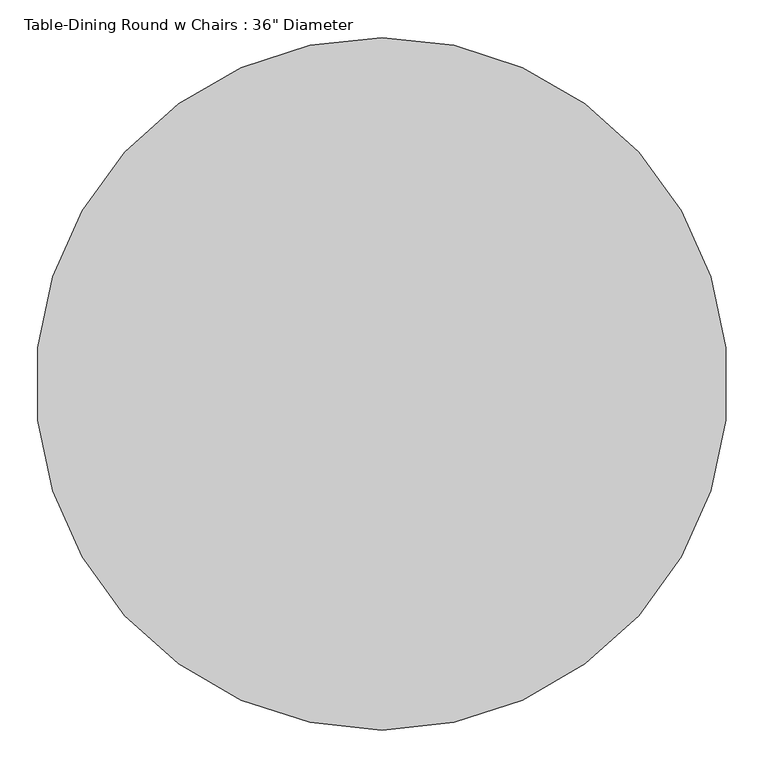
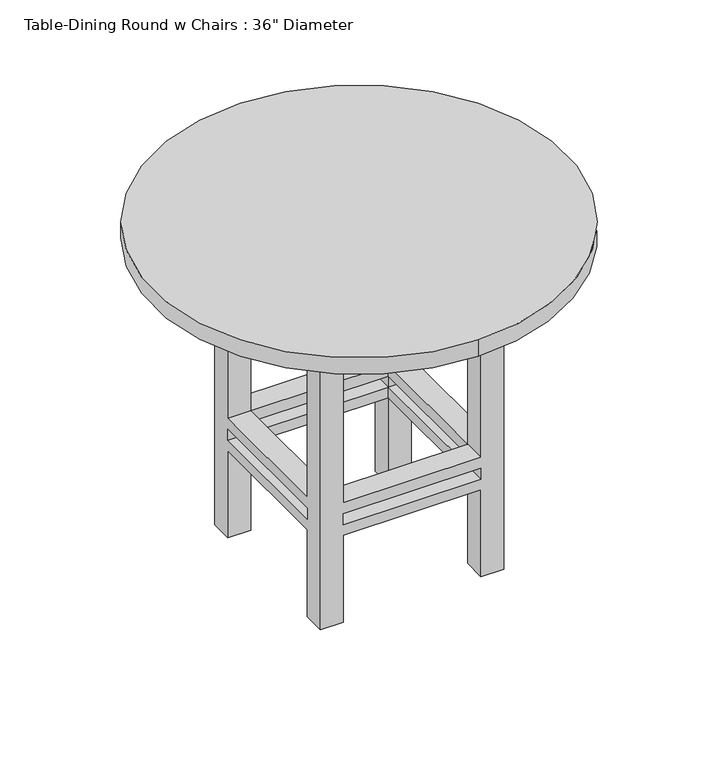
"""IFC4 building model written with IfcOpenShell, lengths in millimetres: furniture geometry."""

from ifc_helpers import new_model, si_unit, point, frame, frame_2d, origin, place, context, project, spatial, polyline, circle_curve, trimmed, segment, composite_curve, outline, extrude, faceted_brep, source, transform, mapped, element, save


def furniture_905aceb5(model_context):
    return source(origin(), model_context, "Body", "SolidModel", [
        faceted_brep([(256.0819672, -32.4786885, 279.4), (256.0819672, -337.2786885, 279.4), (306.8819672, -337.2786885, 279.4), (306.8819672, -32.4786885, 279.4), (-48.7180328, -337.2786885, 279.4), (-48.7180328, -388.0786885, 279.4), (256.0819672, -388.0786885, 279.4), (-48.7180328, -32.4786885, 279.4), (-99.5180328, -32.4786885, 279.4), (-99.5180328, -337.2786885, 279.4), (256.0819672, 18.3213115, 279.4), (-48.7180328, 18.3213115, 279.4), (256.0819672, -32.4786885, 254.0), (-48.7180328, -32.4786885, 254.0), (-48.7180328, 18.3213115, 254.0), (256.0819672, 18.3213115, 254.0), (-48.7180328, -337.2786885, 254.0), (-99.5180328, -337.2786885, 254.0), (-99.5180328, -32.4786885, 254.0), (256.0819672, -337.2786885, 254.0), (256.0819672, -388.0786885, 254.0), (-48.7180328, -388.0786885, 254.0), (306.8819672, -32.4786885, 254.0), (306.8819672, -337.2786885, 254.0), (-99.5180328, 18.3213115, 647.7), (-48.7180328, 18.3213115, 647.7), (256.0819672, 18.3213115, 647.7), (306.8819672, 18.3213115, 647.7), (306.8819672, 18.3213115, 0.0), (256.0819672, 18.3213115, 0.0), (256.0819672, 18.3213115, 203.2), (-48.7180328, 18.3213115, 203.2), (-48.7180328, 18.3213115, 0.0), (-99.5180328, 18.3213115, 0.0), (-48.7180328, 18.3213115, 228.6), (256.0819672, 18.3213115, 228.6), (-99.5180328, -32.4786885, 647.7), (-99.5180328, -32.4786885, 0.0), (-99.5180328, -32.4786885, 203.2), (-99.5180328, -337.2786885, 203.2), (-99.5180328, -337.2786885, 0.0), (-99.5180328, -388.0786885, 0.0), (-99.5180328, -388.0786885, 647.7), (-99.5180328, -337.2786885, 647.7), (-99.5180328, -337.2786885, 228.6), (-99.5180328, -32.4786885, 228.6), (306.8819672, -388.0786885, 647.7), (256.0819672, -388.0786885, 647.7), (-48.7180328, -388.0786885, 647.7), (-48.7180328, -388.0786885, 0.0), (-48.7180328, -388.0786885, 203.2), (256.0819672, -388.0786885, 203.2), (256.0819672, -388.0786885, 0.0), (306.8819672, -388.0786885, 0.0), (256.0819672, -388.0786885, 228.6), (-48.7180328, -388.0786885, 228.6), (306.8819672, -32.4786885, 647.7), (306.8819672, -337.2786885, 647.7), (306.8819672, -337.2786885, 0.0), (306.8819672, -337.2786885, 203.2), (306.8819672, -32.4786885, 203.2), (306.8819672, -32.4786885, 0.0), (306.8819672, -32.4786885, 228.6), (306.8819672, -337.2786885, 228.6), (-48.7180328, -32.4786885, 647.7), (256.0819672, -337.2786885, 647.7), (256.0819672, -32.4786885, 647.7), (-48.7180328, -337.2786885, 647.7), (256.0819672, -32.4786885, 0.0), (-48.7180328, -337.2786885, 0.0), (-48.7180328, -32.4786885, 0.0), (256.0819672, -337.2786885, 0.0), (-48.7180328, -32.4786885, 228.6), (-48.7180328, -32.4786885, 203.2), (256.0819672, -32.4786885, 228.6), (256.0819672, -32.4786885, 203.2), (256.0819672, -337.2786885, 228.6), (256.0819672, -337.2786885, 203.2), (-48.7180328, -337.2786885, 228.6), (-48.7180328, -337.2786885, 203.2)], [[[0, 1, 2, 3]], [[1, 4, 5, 6]], [[4, 7, 8, 9]], [[7, 0, 10, 11]], [[12, 13, 14, 15]], [[13, 16, 17, 18]], [[16, 19, 20, 21]], [[19, 12, 22, 23]], [[24, 25, 11, 10, 26, 27, 28, 29, 30, 31, 32, 33], [14, 34, 35, 15]], [[36, 24, 33, 37, 38, 39, 40, 41, 42, 43, 9, 8], [17, 44, 45, 18]], [[46, 47, 6, 5, 48, 42, 41, 49, 50, 51, 52, 53], [20, 54, 55, 21]], [[28, 27, 56, 3, 2, 57, 46, 53, 58, 59, 60, 61], [22, 62, 63, 23]], [[1, 0, 12, 19]], [[4, 1, 19, 16]], [[7, 4, 16, 13]], [[0, 7, 13, 12]], [[25, 24, 36, 64]], [[47, 46, 57, 65]], [[26, 66, 56, 27]], [[48, 67, 43, 42]], [[29, 28, 61, 68]], [[49, 41, 40, 69]], [[32, 70, 37, 33]], [[52, 71, 58, 53]], [[13, 18, 45, 72]], [[64, 36, 8, 7]], [[37, 70, 73, 38]], [[14, 13, 72, 34]], [[25, 64, 7, 11]], [[70, 32, 31, 73]], [[12, 15, 35, 74]], [[66, 26, 10, 0]], [[29, 68, 75, 30]], [[22, 12, 74, 62]], [[56, 66, 0, 3]], [[68, 61, 60, 75]], [[19, 23, 63, 76]], [[65, 57, 2, 1]], [[58, 71, 77, 59]], [[20, 19, 76, 54]], [[47, 65, 1, 6]], [[71, 52, 51, 77]], [[16, 21, 55, 78]], [[67, 48, 5, 4]], [[49, 69, 79, 50]], [[17, 16, 78, 44]], [[43, 67, 4, 9]], [[69, 40, 39, 79]], [[74, 76, 63, 62]], [[76, 78, 55, 54]], [[78, 72, 45, 44]], [[72, 74, 35, 34]], [[75, 73, 31, 30]], [[73, 79, 39, 38]], [[79, 77, 51, 50]], [[77, 75, 60, 59]], [[76, 74, 75, 77]], [[78, 76, 77, 79]], [[72, 78, 79, 73]], [[74, 72, 73, 75]]]),
        extrude(outline(polyline([(332.2819672, 43.7213115), (332.2819672, -413.4786885), (-124.9180328, -413.4786885), (-124.9180328, 43.7213115), (332.2819672, 43.7213115)]), holes=[polyline([(306.8819672, 18.3213115), (-99.5180328, 18.3213115), (-99.5180328, -388.0786885), (306.8819672, -388.0786885), (306.8819672, 18.3213115)])]), frame((0.0, 0.0, 647.7), z_axis=(0.0, 0.0, 1.0), x_axis=(1.0, 0.0, 0.0)), (0.0, 0.0, 1.0), 76.2),
        extrude(outline(composite_curve([segment(trimmed(circle_curve(frame_2d((103.6819672, -184.8786885)), 457.2), [point((103.6819672, -642.0786885))], [point((103.6819672, 272.3213115))], False, "CARTESIAN"), True, "CONTINUOUS"), segment(trimmed(circle_curve(frame_2d((103.6819672, -184.8786885)), 457.2), [point((103.6819672, 272.3213115))], [point((103.6819672, -642.0786885))], False, "CARTESIAN"), True, "CONTINUOUS")], self_intersect=False)), frame((0.0, 0.0, 723.9), z_axis=(0.0, 0.0, 1.0), x_axis=(1.0, 0.0, 0.0)), (0.0, 0.0, 1.0), 38.1),
    ])


if __name__ == "__main__":
    model = new_model("IFC4")
    model_context = context("Model", 3, world=origin())
    ifc_project = project(units=[si_unit("LENGTHUNIT", "METRE", prefix="MILLI")], contexts=[model_context])
    site = spatial("IfcSite", under=ifc_project)
    building = spatial("IfcBuilding", under=site)
    placement = place(None, origin())
    furniture_shape = furniture_905aceb5(model_context)
    element("IfcFurniture", 1, ObjectType="Table-Dining Round w Chairs : 36\" Diameter", at=placement, inside=building, context=model_context, shape_type="MappedRepresentation", body=[
        mapped(furniture_shape, transform((0.0, 0.0, 0.0), x_axis=(1.0, 0.0, 0.0), y_axis=(0.0, 1.0, 0.0), z_axis=(0.0, 0.0, 1.0))),
    ])
    save(model, "model.ifc")

# Revit data of these elements
# Type "Table-Dining Round w Chairs : 36\" Diameter"
#   Assembly Code = "E2020200"
#   Radius = 1' - 6"
#   Diameter = 3' - 0"
#   Height = 2' - 6"
#   Chairs = 4
#   Base Material = Pine
#   Top Material = Laminate, Linen, Matte
#   Default Elevation = 0
# Element 1 (IfcFurniture, "Table-Dining Round w Chairs : 36\" Diameter")
#   Materials on its faces: "Pine", "Laminate, Linen, Matte"
# Materials
#   "Pine": class "Wood", colour RGB 223 192 134, transparency 0, Description = "Pinus Echinata", Cost = 0
#   "Laminate, Linen, Matte": class "Plastic", colour RGB 249 239 230, transparency 0, Description = "Plastic Laminate - Linen, Matte", Cost = 0
